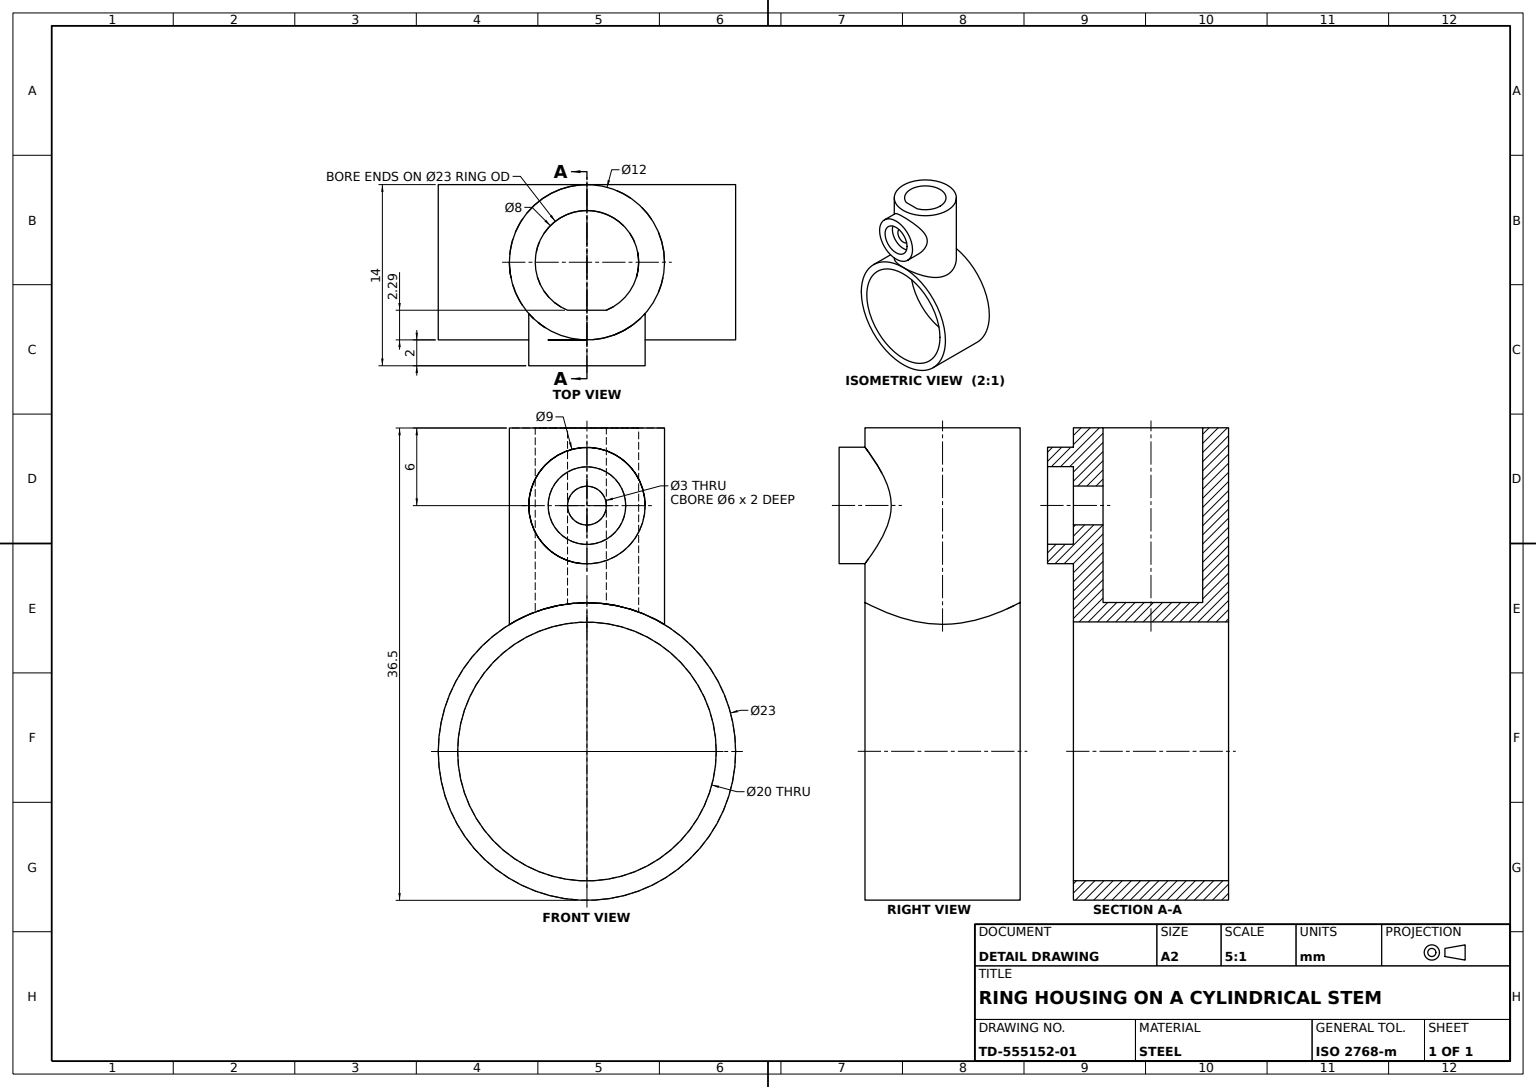
SolidWorks part; units mm, degrees
material "Plain Carbon Steel"
ref_plane "Front Plane" through (0, 0, 0) normal (0, 0, 1) x (1, 0, 0)
ref_plane "Top Plane" through (0, 0, 0) normal (0, 1, 0) x (1, 0, 0)
ref_plane "Right Plane" through (0, 0, 0) normal (1, 0, 0) x (0, 0, -1)
sketch "Ring Profile Ø23-Ø20" plane through (0, 0, 0) normal (0, 0, 1) x (1, 0, 0)
  circle A0 centre (0, 0) radius 10
  circle A1 centre (0, 0) radius 11.5
  dimension "D1" = 20
  dimension "D2" = 23
extrude "Ring Ø23x12" add sketch "Ring Profile Ø23-Ø20" along normal mid plane 12
ref_plane "Plane1" through (0, -25, 0) normal (0, -1, 0) x (-1, 0, 0)
sketch "Stem Profile" plane through (0, -25, 0) normal (0, -1, 0) x (-1, 0, 0)
  line L0 (0, 0) -> (8.4408, 0)
  line L5 (-1.5, -3.7081) -> (1.5, -3.7081)
  circle A0 centre (0, 0) radius 6
  arc A2 (1.5, -3.7081) -> (-1.5, -3.7081) centre (0, 0) ccw
  dimension "D1" = 12
  dimension "D2" = 4
  dimension "D3" = 1.5
  dimension "D4" = 9.9408
extrude "Stem" add sketch "Stem Profile" against normal blind 18
sketch "Ring Cut Profile" plane through (0, 0, 6) normal (0, 0, 1) x (1, 0, 0)
  circle A0 centre (0, 0) radius 10
  dimension "D1" = 20
extrude "Ring Cut" cut sketch "Ring Cut Profile" against normal blind 18
ref_plane "Plane2" through (0, 0, 8) normal (0, 0, 1) x (1, 0, 0)
sketch "Side Boss Profile Ø9" plane through (0, 0, 8) normal (0, 0, 1) x (1, 0, 0)
  line L0 (-7.7, -25) -> (7.7, -25) construction
  circle A2 centre (0, -19) radius 4.5
  dimension "D1" = 9
  dimension "D2" = 6
extrude "Side Boss Ø9" add sketch "Side Boss Profile Ø9" against normal blind 6
sketch "Side Hole Profile Ø3" plane through (0, 0, 8) normal (0, 0, 1) x (1, 0, 0)
  circle A0 centre (0, -19) radius 1.5
  dimension "D1" = 3
extrude "Side Hole Ø3" cut sketch "Side Hole Profile Ø3" against normal blind 6
sketch "Counterbore Profile Ø6" plane through (0, 0, 8) normal (0, 0, 1) x (1, 0, 0)
  circle A0 centre (0, -19) radius 3
  circle A1 centre (0, -19) radius 1.5
  dimension "D1" = 6
  dimension "D2" = 3
extrude "Counterbore Ø6x2" cut sketch "Counterbore Profile Ø6" against normal blind 2
sketch "Stem Trim Profile" plane through (0, -25, 0) normal (0, -1, 0) x (1, 0, 0)
  line L0 (-1.2398, 3.7081) -> (-1.5, 3.7081)
  line L1 (-1.5, 3.7081) -> (1.5, 3.7081) construction
  line L2 (-1.5, 3.7081) -> (1.5, 3.7081)
  arc A0 (-1.5, 3.7081) -> (1.5, 3.7081) centre (0, 0) ccw
  dimension "D1" = 0.2602
extrude "Stem Trim Cut" cut sketch "Stem Trim Profile" against normal blind 12 contours A0 L2
